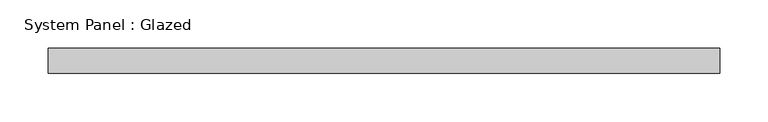
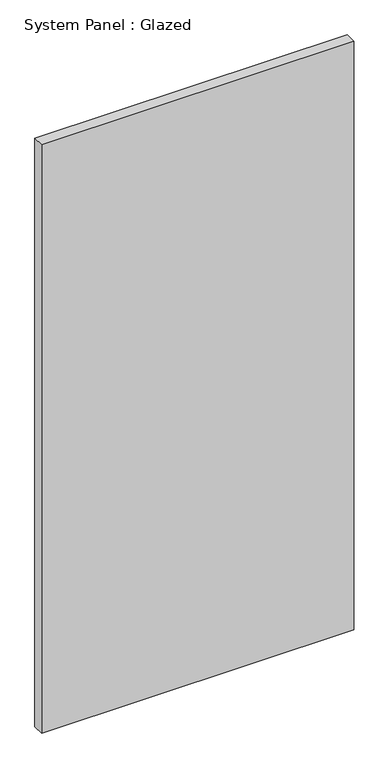
"""IFC4 building model written with IfcOpenShell, lengths in millimetres: plate geometry, System Panel : Glazed."""

from ifc_helpers import new_model, si_unit, origin, origin_with_axes, place, context, project, spatial, polyline, outline, extrude, source, transform, mapped, element, save


def system_panel_glazed_d353ffa9(model_context):
    return source(origin(), model_context, "Body", "SweptSolid", [
        extrude(outline(polyline([(346.075, 19.05), (-346.075, 19.05), (-346.075, 44.45), (346.075, 44.45), (346.075, 19.05)])), origin_with_axes(), (0.0, 0.0, 1.0), 1379.17602),
    ])


if __name__ == "__main__":
    model = new_model("IFC4")
    model_context = context("Model", 3, world=origin())
    ifc_project = project(units=[si_unit("LENGTHUNIT", "METRE", prefix="MILLI")], contexts=[model_context])
    site = spatial("IfcSite", under=ifc_project)
    building = spatial("IfcBuilding", under=site)
    placement = place(None, origin())
    system_panel_glazed_shape = system_panel_glazed_d353ffa9(model_context)
    element("IfcPlate", 1, ObjectType="System Panel : Glazed", at=placement, inside=building, context=model_context, shape_type="MappedRepresentation", body=[
        mapped(system_panel_glazed_shape, transform((0.0, 0.0, 0.0), x_axis=(1.0, 0.0, 0.0), y_axis=(0.0, 1.0, 0.0), z_axis=(0.0, 0.0, 1.0))),
    ])
    save(model, "model.ifc")

# Revit data of these elements
# Type "System Panel : Glazed"
#   Construction Type Id = "GSP4R"
#   Analytic Construction = "1/8 in Pilkington single glazing"
#   Visual Light Transmittance = 0.9
#   Solar Heat Gain Coefficient = 0.86
#   Heat Transfer Coefficient (U) = 1.18115 BTU/(h·ft²·°F)
#   Define Thermal Properties by = 1
# Element 1 (IfcPlate, "System Panel : Glazed")
#   Materials on its faces: "Glass"
# Materials
#   "Glass": class "Glass", colour RGB 0 128 192, transparency 0.75, Description = "Soda Lime Glass", Cost = 0
